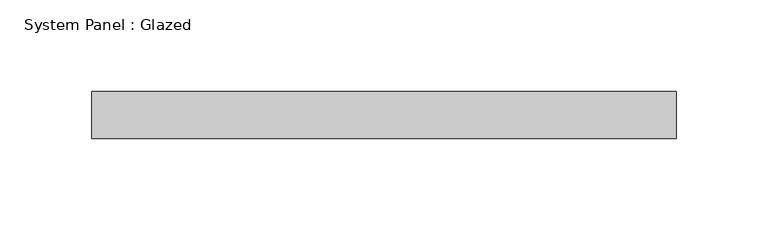
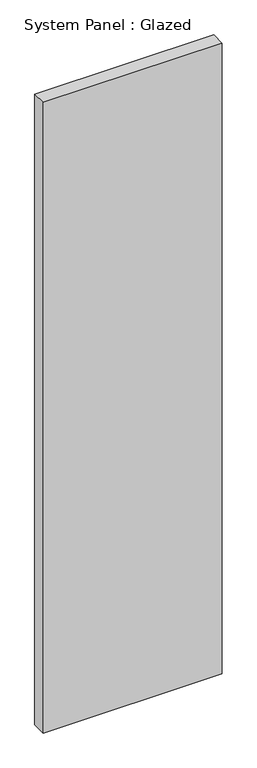
"""IFC4 building model written with IfcOpenShell, lengths in millimetres: plate geometry, System Panel : Glazed."""

from ifc_helpers import new_model, si_unit, origin, origin_with_axes, place, context, project, spatial, polyline, outline, extrude, source, transform, mapped, element, save


def system_panel_glazed_de0a1ab2(model_context):
    return source(origin(), model_context, "Body", "SweptSolid", [
        extrude(outline(polyline([(158.75, 19.05), (-158.75, 19.05), (-158.75, 44.45), (158.75, 44.45), (158.75, 19.05)])), origin_with_axes(), (0.0, 0.0, 1.0), 1181.1),
    ])


if __name__ == "__main__":
    model = new_model("IFC4")
    model_context = context("Model", 3, world=origin())
    ifc_project = project(units=[si_unit("LENGTHUNIT", "METRE", prefix="MILLI")], contexts=[model_context])
    site = spatial("IfcSite", under=ifc_project)
    building = spatial("IfcBuilding", under=site)
    placement = place(None, origin())
    system_panel_glazed_shape = system_panel_glazed_de0a1ab2(model_context)
    element("IfcPlate", 1, ObjectType="System Panel : Glazed", at=placement, inside=building, context=model_context, shape_type="MappedRepresentation", body=[
        mapped(system_panel_glazed_shape, transform((0.0, 0.0, 0.0), x_axis=(1.0, 0.0, 0.0), y_axis=(0.0, 1.0, 0.0), z_axis=(0.0, 0.0, 1.0))),
    ])
    save(model, "model.ifc")

# Revit data of these elements
# Type "System Panel : Glazed"
#   Construction Type Id = "GSP4R"
#   Analytic Construction = "1/8 in Pilkington single glazing"
#   Visual Light Transmittance = 0.9
#   Solar Heat Gain Coefficient = 0.86
#   Heat Transfer Coefficient (U) = 1.18115 BTU/(h·ft²·°F)
#   Define Thermal Properties by = 1
# Element 1 (IfcPlate, "System Panel : Glazed")
#   Materials on its faces: "Glass"
# Materials
#   "Glass": class "Glass", colour RGB 0 128 192, transparency 0.75, Description = "Soda Lime Glass", Cost = 0
